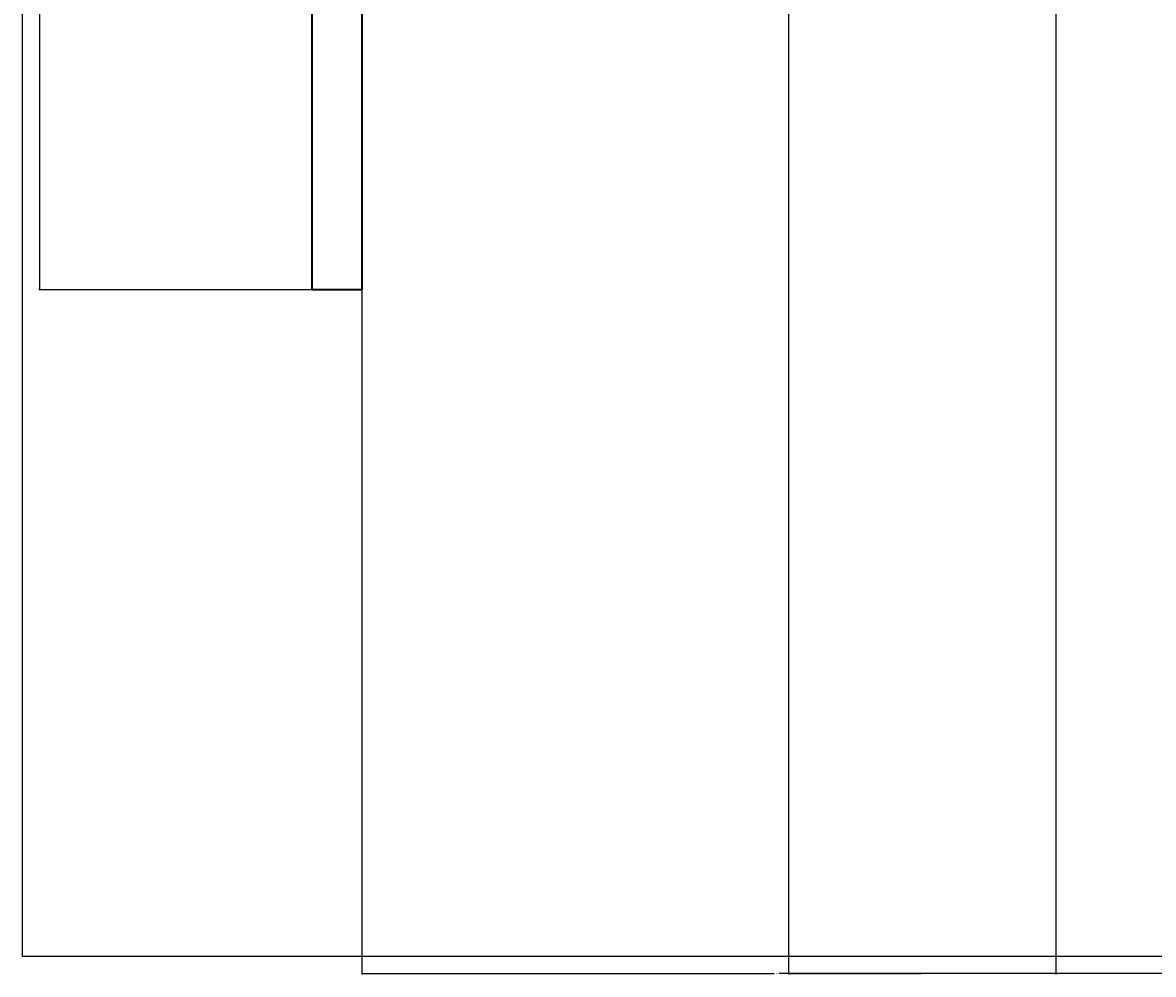
# Model space of a CAD drawing. Units: inches. Extents: x 2460 to 3031, y 933 to 2010.
# Tile 1 of 7: x 2460 to 2663, y 933 to 1104. Entities that reach past the tile are written whole.
import ezdxf

# ---------------------------------------------------------------- set-up
doc = ezdxf.new("R2010")
doc.units = ezdxf.units.IN
for name, color, linetype, lineweight in [('A-ANNO-DIMS', 2, 'Continuous', 18), ('A-ANNO-TTLB', 7, 'Continuous', 25), ('C-PROP', 7, 'Continuous', 35)]:
    doc.layers.add(name, color=color, linetype=linetype, lineweight=lineweight)
doc.styles.get("Standard").update_dxf_attribs({"font": 'arial.ttf'})
doc.dimstyles.get("Standard").update_dxf_attribs({"dimtxt": 0.18, "dimasz": 0.18, "dimexe": 0.18, "dimexo": 0.0625, "dimgap": 0.09, "dimtad": 0, "dimtih": 1, "dimtoh": 1, "dimdec": 4, "dimzin": 0, "dimdsep": 46, "dimtxsty": 'Standard', "dimcen": 0.09, "dimadec": 0, "dimazin": 0, "dimtfac": 1, "dimtdec": 4, "dimtofl": 0, "dimtmove": 0, "dimatfit": 3, "dimfxl": 1, "dimtolj": 1, "dimtzin": 0, "dimarcsym": 0})

# ---------------------------------------------------------------- blocks, each defined once
blk = doc.blocks.new('*D34')
at = {"layer": 'A-ANNO-DIMS', "color": 0, "lineweight": -2, "transparency": 16777216}
for p, q in [((2520.67, 1055.92), (2520.67, 933.16)), ((2669.43, 1055.92), (2669.43, 933.16)), ((2520.85, 933.34), (2594.6, 933.34)), ((2669.25, 933.34), (2595.51, 933.34))]:
    blk.add_line(p, q, dxfattribs=at)
at = {"layer": 'A-ANNO-DIMS', "color": 0, "transparency": 16777216}
for points in [[(2520.85, 933.37), (2520.85, 933.31), (2520.67, 933.34)], [(2669.25, 933.37), (2669.25, 933.31), (2669.43, 933.34)]]:
    blk.add_solid(points, dxfattribs=at)
at = {"layer": 'Defpoints', "color": 0, "transparency": 16777216}
for p in [(2520.67, 1055.98), (2669.43, 1055.98), (2669.43, 933.34)]:
    blk.add_point(p, dxfattribs=at)
at = {"layer": 'A-ANNO-DIMS', "color": 0, "transparency": 16777216, "insert": (2595.05, 933.34), "char_height": 0.18, "attachment_point": 5}
blk.add_mtext('\\A1;148.76', dxfattribs=at)
blk = doc.blocks.new('*D35')
at = {"layer": 'A-ANNO-DIMS', "color": 0, "lineweight": -2, "transparency": 16777216}
for p, q in [((2520.61, 1339.48), (2462.69, 1339.48)), ((2462.87, 1339.3), (2462.87, 1197.91)), ((2462.87, 1056.16), (2462.87, 1197.55)), ((2511.61, 1055.98), (2462.69, 1055.98))]:
    blk.add_line(p, q, dxfattribs=at)
at = {"layer": 'A-ANNO-DIMS', "color": 0, "transparency": 16777216}
for points in [[(2462.84, 1339.3), (2462.9, 1339.3), (2462.87, 1339.48)], [(2462.84, 1056.16), (2462.9, 1056.16), (2462.87, 1055.98)]]:
    blk.add_solid(points, dxfattribs=at)
at = {"layer": 'Defpoints', "color": 0, "transparency": 16777216}
for p in [(2462.87, 1339.48), (2520.67, 1339.48), (2511.67, 1055.98)]:
    blk.add_point(p, dxfattribs=at)
at = {"layer": 'A-ANNO-DIMS', "color": 0, "transparency": 16777216, "insert": (2462.87, 1197.73), "char_height": 0.18, "attachment_point": 5}
blk.add_mtext('\\A1;283.5', dxfattribs=at)
blk = doc.blocks.new('*D37')
at = {"layer": 'A-ANNO-DIMS', "color": 0, "lineweight": -2, "transparency": 16777216}
for p, q in [((2597.17, 1554.98), (2597.17, 933.16)), ((2645.17, 1554.98), (2645.17, 933.16)), ((2597.35, 933.34), (2620.95, 933.34)), ((2644.99, 933.34), (2621.39, 933.34))]:
    blk.add_line(p, q, dxfattribs=at)
at = {"layer": 'A-ANNO-DIMS', "color": 0, "transparency": 16777216}
for points in [[(2597.35, 933.37), (2597.35, 933.31), (2597.17, 933.34)], [(2644.99, 933.37), (2644.99, 933.31), (2645.17, 933.34)]]:
    blk.add_solid(points, dxfattribs=at)
at = {"layer": 'Defpoints', "color": 0, "transparency": 16777216}
for p in [(2597.17, 1555.05), (2645.17, 1555.05), (2645.17, 933.34)]:
    blk.add_point(p, dxfattribs=at)
at = {"layer": 'A-ANNO-DIMS', "color": 0, "transparency": 16777216, "insert": (2621.17, 933.34), "char_height": 0.18, "attachment_point": 5}
blk.add_mtext('\\A1;48', dxfattribs=at)
blk = doc.blocks.new('*D40')
at = {"layer": 'A-ANNO-DIMS', "color": 0, "lineweight": -2, "transparency": 16777216}
for p, q in [((2511.67, 1056.05), (2511.67, 2006.96)), ((2511.85, 2006.78), (2516.02, 2006.78)), ((2520.49, 2006.78), (2516.32, 2006.78)), ((2520.67, 1056.05), (2520.67, 2006.96))]:
    blk.add_line(p, q, dxfattribs=at)
at = {"layer": 'A-ANNO-DIMS', "color": 0, "transparency": 16777216}
for points in [[(2511.85, 2006.81), (2511.85, 2006.75), (2511.67, 2006.78)], [(2520.49, 2006.81), (2520.49, 2006.75), (2520.67, 2006.78)]]:
    blk.add_solid(points, dxfattribs=at)
at = {"layer": 'Defpoints', "color": 0, "transparency": 16777216}
for p in [(2520.67, 2006.78), (2511.67, 1055.98), (2520.67, 1055.98)]:
    blk.add_point(p, dxfattribs=at)
at = {"layer": 'A-ANNO-DIMS', "color": 0, "transparency": 16777216, "insert": (2516.17, 2006.78), "char_height": 0.18, "attachment_point": 5}
blk.add_mtext('\\A1;9', dxfattribs=at)

msp = doc.modelspace()

# ---------------------------------------------------------------- linework, layer by layer
at = {"layer": 'A-ANNO-TTLB'}
msp.add_lwpolyline([(2459.8083, 2009.7942), (3030.6598, 2009.7942), (3030.6598, 936.3732), (2459.8083, 936.3732)], close=True, dxfattribs=at)
at = {"layer": 'C-PROP'}
for p, q in [((2511.6684, 1957.9828), (2511.6684, 1055.9828)), ((2511.6684, 1957.9828), (2511.6684, 1055.9828)), ((2520.6684, 1339.4828), (2520.6684, 1055.9828)), ((2520.6684, 1055.9828), (2511.6684, 1055.9828))]:
    msp.add_line(p, q, dxfattribs=at)

# ---------------------------------------------------------------- dimensions: what is measured, and where the dimension line sits
at = {"layer": 'A-ANNO-DIMS'}
for base, p1, p2, override, picture, middle in [((2520.6684, 2006.7823), (2511.6684, 1055.9828), (2520.6684, 1055.9828), {"dimdec": 0, "dimlfac": 1, "dimrnd": 0, "dimzin": 0, "dimdsep": 46, "dimlunit": 2}, '*D40', (2516.1684, 2006.7823)), ((2645.1684, 933.3411), (2597.1684, 1555.0454), (2645.1684, 1555.0454), {"dimdec": 0, "dimlfac": 1, "dimrnd": 0, "dimzin": 0, "dimdsep": 46, "dimlunit": 2}, '*D37', (2621.1684, 933.3411)), ((2669.433, 933.3411), (2520.6684, 1055.9828), (2669.433, 1055.9828), {"dimdec": 2, "dimlfac": 1, "dimrnd": 0, "dimzin": 0, "dimdsep": 46, "dimlunit": 2}, '*D34', (2595.0507, 933.3411))]:
    dim = msp.add_linear_dim(base=base, p1=p1, p2=p2, dimstyle='Standard', override=override, dxfattribs=at)
    dim.commit()
    dim.dimension.update_dxf_attribs({"geometry": picture, "text_midpoint": middle})
dim = msp.add_linear_dim(base=(2462.8689, 1339.4828), p1=(2511.6684, 1055.9828), p2=(2520.6684, 1339.4828), angle=90, dimstyle='Standard', override={"dimdec": 1, "dimlfac": 1, "dimrnd": 0, "dimzin": 0, "dimdsep": 46, "dimlunit": 2}, dxfattribs=at)
dim.commit()
dim.dimension.update_dxf_attribs({"geometry": '*D35', "text_midpoint": (2462.8689, 1197.7328)})

doc.saveas('drawing.dxf')
